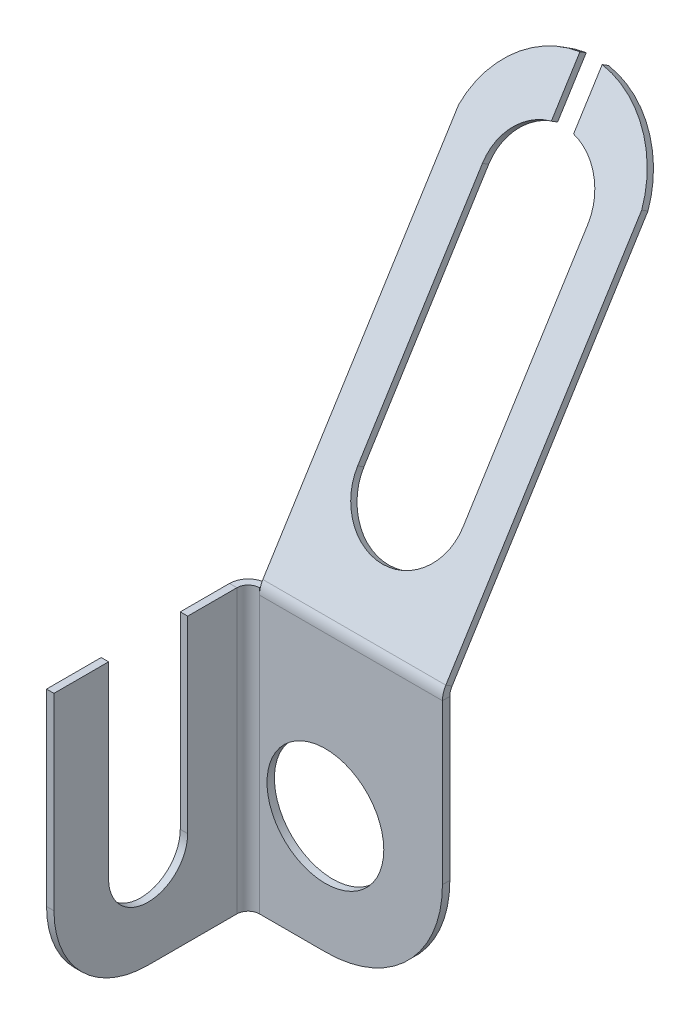
ISO-10303-21;
HEADER;
FILE_DESCRIPTION(('STEP AP214'),'2;1');
FILE_NAME('part.step','',(''),(''),'','','');
FILE_SCHEMA(('AUTOMOTIVE_DESIGN { 1 0 10303 214 1 1 1 1 }'));
ENDSEC;
DATA;
#1=APPLICATION_CONTEXT('core data for automotive mechanical design processes');
#2=APPLICATION_PROTOCOL_DEFINITION('international standard','automotive_design',2000,#1);
#3=PRODUCT_CONTEXT('',#1,'mechanical');
#4=PRODUCT('Part','Part','',(#3));
#5=PRODUCT_RELATED_PRODUCT_CATEGORY('part','',(#4));
#6=PRODUCT_DEFINITION_FORMATION('','',#4);
#7=PRODUCT_DEFINITION_CONTEXT('part definition',#1,'design');
#8=PRODUCT_DEFINITION('design','',#6,#7);
#9=PRODUCT_DEFINITION_SHAPE('','',#8);
#10=(LENGTH_UNIT() NAMED_UNIT(*) SI_UNIT(.MILLI.,.METRE.));
#11=(NAMED_UNIT(*) PLANE_ANGLE_UNIT() SI_UNIT($,.RADIAN.));
#12=(NAMED_UNIT(*) SI_UNIT($,.STERADIAN.) SOLID_ANGLE_UNIT());
#13=UNCERTAINTY_MEASURE_WITH_UNIT(LENGTH_MEASURE(1.E-05),#10,'distance_accuracy_value','');
#14=(GEOMETRIC_REPRESENTATION_CONTEXT(3) GLOBAL_UNCERTAINTY_ASSIGNED_CONTEXT((#13)) GLOBAL_UNIT_ASSIGNED_CONTEXT((#10,
#11,#12)) REPRESENTATION_CONTEXT('',''));
#15=CARTESIAN_POINT('',(0.,0.,0.));
#16=DIRECTION('',(0.,0.,1.));
#17=DIRECTION('',(1.,0.,0.));
#18=AXIS2_PLACEMENT_3D('',#15,#16,#17);
#19=CARTESIAN_POINT('',(1.25999999999999,55.0512584693438,-34.2878670812797));
#20=DIRECTION('',(0.,0.5299192642332,0.848048096156429));
#21=DIRECTION('',(0.,-0.848048096156429,0.5299192642332));
#22=AXIS2_PLACEMENT_3D('',#19,#20,#21);
#23=CYLINDRICAL_SURFACE('',#22,12.5);
#24=DIRECTION('',(0.,0.5299192642332,0.848048096156429));
#25=VECTOR('',#24,1.);
#26=CARTESIAN_POINT('',(2.76000000000004,65.5752585787489,-40.8639922091373));
#27=LINE('',#26,#25);
#28=CARTESIAN_POINT('',(2.76000000000004,70.3445319568478,-33.2315593437294));
#29=VERTEX_POINT('',#28);
#30=CARTESIAN_POINT('',(2.76000000000004,70.8744512210809,-32.383511247573));
#31=VERTEX_POINT('',#30);
#32=EDGE_CURVE('E289',#29,#31,#27,.T.);
#33=ORIENTED_EDGE('',*,*,#32,.T.);
#34=CARTESIAN_POINT('',(1.25999999999999,60.3504511116758,-25.8073861197154));
#35=DIRECTION('',(0.,0.5299192642332,0.848048096156429));
#36=DIRECTION('',(0.,-0.848048096156429,0.5299192642332));
#37=AXIS2_PLACEMENT_3D('',#34,#35,#36);
#38=CIRCLE('',#37,12.5);
#39=CARTESIAN_POINT('',(13.5977,62.0531405103318,-26.8713445407565));
#40=VERTEX_POINT('',#39);
#41=EDGE_CURVE('E302',#40,#31,#38,.T.);
#42=ORIENTED_EDGE('',*,*,#41,.F.);
#43=DIRECTION('',(0.,0.5299192642332,0.848048096156429));
#44=VECTOR('',#43,1.);
#45=CARTESIAN_POINT('',(13.5977,56.7539478679998,-35.3518255023207));
#46=LINE('',#45,#44);
#47=CARTESIAN_POINT('',(13.5977,61.5232212460986,-27.7193926369129));
#48=VERTEX_POINT('',#47);
#49=EDGE_CURVE('E310',#48,#40,#46,.T.);
#50=ORIENTED_EDGE('',*,*,#49,.F.);
#51=CARTESIAN_POINT('',(1.25999999999999,59.8205318474426,-26.6554342158718));
#52=DIRECTION('',(0.,0.5299192642332,0.848048096156429));
#53=DIRECTION('',(0.,-0.848048096156429,0.5299192642332));
#54=AXIS2_PLACEMENT_3D('',#51,#52,#53);
#55=CIRCLE('',#54,12.5);
#56=EDGE_CURVE('E314',#48,#29,#55,.T.);
#57=ORIENTED_EDGE('',*,*,#56,.T.);
#58=EDGE_LOOP('',(#33,#42,#50,#57));
#59=FACE_BOUND('',#58,.T.);
#60=ADVANCED_FACE('F103',(#59),#23,.T.);
#61=CARTESIAN_POINT('',(1.25999999999998,53.5052484421712,-33.321812797555));
#62=DIRECTION('',(0.,0.5299192642332,0.848048096156429));
#63=DIRECTION('',(0.,-0.848048096156429,0.5299192642332));
#64=AXIS2_PLACEMENT_3D('',#61,#62,#63);
#65=CYLINDRICAL_SURFACE('',#64,7.112);
#66=CARTESIAN_POINT('',(1.25999999999998,58.8044410845032,-24.8413318359907));
#67=DIRECTION('',(0.,0.5299192642332,0.848048096156429));
#68=DIRECTION('',(0.,-0.848048096156429,0.5299192642332));
#69=AXIS2_PLACEMENT_3D('',#66,#67,#68);
#70=CIRCLE('',#69,7.112);
#71=CARTESIAN_POINT('',(8.37199999999998,58.8044410845032,-24.8413318359907));
#72=VERTEX_POINT('',#71);
#73=CARTESIAN_POINT('',(2.76000000000004,64.7000860873091,-28.5253397079815));
#74=VERTEX_POINT('',#73);
#75=EDGE_CURVE('E504',#72,#74,#70,.T.);
#76=ORIENTED_EDGE('',*,*,#75,.T.);
#77=DIRECTION('',(0.,0.5299192642332,0.848048096156429));
#78=VECTOR('',#77,1.);
#79=CARTESIAN_POINT('',(2.76000000000004,59.4008934449771,-37.0058206695458));
#80=LINE('',#79,#78);
#81=CARTESIAN_POINT('',(2.76000000000004,64.1701668230759,-29.3733878041379));
#82=VERTEX_POINT('',#81);
#83=EDGE_CURVE('E13',#74,#82,#80,.F.);
#84=ORIENTED_EDGE('',*,*,#83,.T.);
#85=CARTESIAN_POINT('',(1.25999999999998,58.27452182027,-25.6893799321472));
#86=DIRECTION('',(0.,0.5299192642332,0.848048096156429));
#87=DIRECTION('',(0.,-0.848048096156429,0.5299192642332));
#88=AXIS2_PLACEMENT_3D('',#85,#86,#87);
#89=CIRCLE('',#88,7.112);
#90=CARTESIAN_POINT('',(8.37199999999998,58.27452182027,-25.6893799321472));
#91=VERTEX_POINT('',#90);
#92=EDGE_CURVE('E489',#91,#82,#89,.T.);
#93=ORIENTED_EDGE('',*,*,#92,.F.);
#94=DIRECTION('',(0.,0.5299192642332,0.848048096156429));
#95=VECTOR('',#94,1.);
#96=CARTESIAN_POINT('',(8.37199999999998,53.5052484421712,-33.321812797555));
#97=LINE('',#96,#95);
#98=EDGE_CURVE('E308',#91,#72,#97,.T.);
#99=ORIENTED_EDGE('',*,*,#98,.T.);
#100=EDGE_LOOP('',(#76,#84,#93,#99));
#101=FACE_BOUND('',#100,.T.);
#102=ADVANCED_FACE('F533',(#101),#65,.F.);
#103=CARTESIAN_POINT('',(0.,5.14329168215875,8.6898758137614));
#104=DIRECTION('',(0.,0.5299192642332,0.848048096156429));
#105=DIRECTION('',(0.,-0.848048096156429,0.5299192642332));
#106=AXIS2_PLACEMENT_3D('',#103,#104,#105);
#107=PLANE('',#106);
#108=DIRECTION('',(0.,0.848048096156429,-0.5299192642332));
#109=VECTOR('',#108,1.);
#110=CARTESIAN_POINT('',(2.76000000000004,70.8744512210809,-32.383511247573));
#111=LINE('',#110,#109);
#112=EDGE_CURVE('E287',#74,#31,#111,.T.);
#113=ORIENTED_EDGE('',*,*,#112,.F.);
#114=ORIENTED_EDGE('',*,*,#75,.F.);
#115=DIRECTION('',(0.,0.848048096156429,-0.5299192642332));
#116=VECTOR('',#115,1.);
#117=CARTESIAN_POINT('',(8.37199999999998,58.8044410845032,-24.8413318359907));
#118=LINE('',#117,#116);
#119=CARTESIAN_POINT('',(8.37199999999999,31.8789140315366,-8.01639519658663));
#120=VERTEX_POINT('',#119);
#121=EDGE_CURVE('E511',#120,#72,#118,.T.);
#122=ORIENTED_EDGE('',*,*,#121,.F.);
#123=CARTESIAN_POINT('',(1.25999999999999,31.8789140315366,-8.01639519658663));
#124=DIRECTION('',(0.,0.5299192642332,0.848048096156429));
#125=DIRECTION('',(0.,-0.848048096156429,0.5299192642332));
#126=AXIS2_PLACEMENT_3D('',#123,#124,#125);
#127=CIRCLE('',#126,7.112);
#128=CARTESIAN_POINT('',(-5.85200000000001,31.8789140315366,-8.01639519658663));
#129=VERTEX_POINT('',#128);
#130=EDGE_CURVE('E512',#129,#120,#127,.T.);
#131=ORIENTED_EDGE('',*,*,#130,.F.);
#132=DIRECTION('',(0.,-0.848048096156429,0.5299192642332));
#133=VECTOR('',#132,1.);
#134=CARTESIAN_POINT('',(-5.85200000000002,58.8044410845032,-24.8413318359907));
#135=LINE('',#134,#133);
#136=CARTESIAN_POINT('',(-5.85200000000002,58.8044410845032,-24.8413318359907));
#137=VERTEX_POINT('',#136);
#138=EDGE_CURVE('E507',#137,#129,#135,.T.);
#139=ORIENTED_EDGE('',*,*,#138,.F.);
#140=CARTESIAN_POINT('',(-0.239999999999953,64.7000860873091,-28.5253397079815));
#141=VERTEX_POINT('',#140);
#142=EDGE_CURVE('E296',#141,#137,#70,.T.);
#143=ORIENTED_EDGE('',*,*,#142,.F.);
#144=DIRECTION('',(0.,-0.848048096156429,0.5299192642332));
#145=VECTOR('',#144,1.);
#146=CARTESIAN_POINT('',(-0.239999999999957,70.874451221081,-32.383511247573));
#147=LINE('',#146,#145);
#148=CARTESIAN_POINT('',(-0.239999999999957,70.874451221081,-32.383511247573));
#149=VERTEX_POINT('',#148);
#150=EDGE_CURVE('E124',#149,#141,#147,.T.);
#151=ORIENTED_EDGE('',*,*,#150,.F.);
#152=CARTESIAN_POINT('',(-11.0777,62.0531405103319,-26.8713445407565));
#153=VERTEX_POINT('',#152);
#154=EDGE_CURVE('E294',#149,#153,#38,.T.);
#155=ORIENTED_EDGE('',*,*,#154,.T.);
#156=DIRECTION('',(0.,0.848048096156429,-0.5299192642332));
#157=VECTOR('',#156,1.);
#158=CARTESIAN_POINT('',(-11.0777,70.9510523136312,-32.4313769226304));
#159=LINE('',#158,#157);
#160=CARTESIAN_POINT('',(-11.0777,19.7795216354232,-0.455855711530713));
#161=VERTEX_POINT('',#160);
#162=EDGE_CURVE('E325',#161,#153,#159,.T.);
#163=ORIENTED_EDGE('',*,*,#162,.F.);
#164=DIRECTION('',(1.,0.,0.));
#165=VECTOR('',#164,1.);
#166=CARTESIAN_POINT('',(0.,19.7795216354232,-0.455855711530716));
#167=LINE('',#166,#165);
#168=CARTESIAN_POINT('',(13.5977,19.7795216354232,-0.455855711530714));
#169=VERTEX_POINT('',#168);
#170=EDGE_CURVE('E329',#161,#169,#167,.T.);
#171=ORIENTED_EDGE('',*,*,#170,.T.);
#172=DIRECTION('',(0.,-0.848048096156429,0.5299192642332));
#173=VECTOR('',#172,1.);
#174=CARTESIAN_POINT('',(13.5977,19.2931738784744,-0.151951903843572));
#175=LINE('',#174,#173);
#176=EDGE_CURVE('E316',#40,#169,#175,.T.);
#177=ORIENTED_EDGE('',*,*,#176,.F.);
#178=ORIENTED_EDGE('',*,*,#41,.T.);
#179=EDGE_LOOP('',(#113,#114,#122,#131,#139,#143,#151,#155,#163,#171,#177,#178));
#180=FACE_BOUND('',#179,.T.);
#181=ADVANCED_FACE('F291',(#180),#107,.T.);
#182=CARTESIAN_POINT('',(0.,4.61337241792555,7.84182771760497));
#183=DIRECTION('',(0.,0.5299192642332,0.848048096156429));
#184=DIRECTION('',(0.,-0.848048096156429,0.5299192642332));
#185=AXIS2_PLACEMENT_3D('',#182,#183,#184);
#186=PLANE('',#185);
#187=ORIENTED_EDGE('',*,*,#92,.T.);
#188=DIRECTION('',(0.,0.848048096156429,-0.5299192642332));
#189=VECTOR('',#188,1.);
#190=CARTESIAN_POINT('',(2.76000000000004,4.61337241792555,7.84182771760497));
#191=LINE('',#190,#189);
#192=EDGE_CURVE('E116',#82,#29,#191,.T.);
#193=ORIENTED_EDGE('',*,*,#192,.T.);
#194=ORIENTED_EDGE('',*,*,#56,.F.);
#195=DIRECTION('',(0.,0.848048096156429,-0.5299192642332));
#196=VECTOR('',#195,1.);
#197=CARTESIAN_POINT('',(13.5977,4.61337241792555,7.84182771760497));
#198=LINE('',#197,#196);
#199=CARTESIAN_POINT('',(13.5977,19.24960237119,-1.30390380768714));
#200=VERTEX_POINT('',#199);
#201=EDGE_CURVE('E323',#48,#200,#198,.F.);
#202=ORIENTED_EDGE('',*,*,#201,.T.);
#203=DIRECTION('',(-1.,0.,0.));
#204=VECTOR('',#203,1.);
#205=CARTESIAN_POINT('',(-11.0777,19.24960237119,-1.30390380768714));
#206=LINE('',#205,#204);
#207=CARTESIAN_POINT('',(-11.0777,19.24960237119,-1.30390380768714));
#208=VERTEX_POINT('',#207);
#209=EDGE_CURVE('E334',#208,#200,#206,.F.);
#210=ORIENTED_EDGE('',*,*,#209,.F.);
#211=DIRECTION('',(0.,-0.848048096156429,0.5299192642332));
#212=VECTOR('',#211,1.);
#213=CARTESIAN_POINT('',(-11.0777,4.61337241792555,7.84182771760497));
#214=LINE('',#213,#212);
#215=CARTESIAN_POINT('',(-11.0777,61.5232212460987,-27.7193926369129));
#216=VERTEX_POINT('',#215);
#217=EDGE_CURVE('E328',#208,#216,#214,.F.);
#218=ORIENTED_EDGE('',*,*,#217,.T.);
#219=CARTESIAN_POINT('',(-0.239999999999957,70.3445319568478,-33.2315593437294));
#220=VERTEX_POINT('',#219);
#221=EDGE_CURVE('E313',#220,#216,#55,.T.);
#222=ORIENTED_EDGE('',*,*,#221,.F.);
#223=DIRECTION('',(0.,-0.848048096156429,0.5299192642332));
#224=VECTOR('',#223,1.);
#225=CARTESIAN_POINT('',(-0.239999999999957,4.61337241792555,7.84182771760497));
#226=LINE('',#225,#224);
#227=CARTESIAN_POINT('',(-0.239999999999952,64.1701668230759,-29.3733878041379));
#228=VERTEX_POINT('',#227);
#229=EDGE_CURVE('E282',#220,#228,#226,.T.);
#230=ORIENTED_EDGE('',*,*,#229,.T.);
#231=CARTESIAN_POINT('',(-5.85200000000002,58.27452182027,-25.6893799321471));
#232=VERTEX_POINT('',#231);
#233=EDGE_CURVE('E490',#228,#232,#89,.T.);
#234=ORIENTED_EDGE('',*,*,#233,.T.);
#235=DIRECTION('',(0.,-0.848048096156429,0.5299192642332));
#236=VECTOR('',#235,1.);
#237=CARTESIAN_POINT('',(-5.852,4.61337241792555,7.84182771760497));
#238=LINE('',#237,#236);
#239=CARTESIAN_POINT('',(-5.85200000000001,31.3489947673034,-8.86444329274306));
#240=VERTEX_POINT('',#239);
#241=EDGE_CURVE('E476',#232,#240,#238,.T.);
#242=ORIENTED_EDGE('',*,*,#241,.T.);
#243=CARTESIAN_POINT('',(1.25999999999999,31.3489947673034,-8.86444329274305));
#244=DIRECTION('',(0.,0.5299192642332,0.848048096156429));
#245=DIRECTION('',(0.,-0.848048096156429,0.5299192642332));
#246=AXIS2_PLACEMENT_3D('',#243,#244,#245);
#247=CIRCLE('',#246,7.112);
#248=CARTESIAN_POINT('',(8.37199999999999,31.3489947673034,-8.86444329274306));
#249=VERTEX_POINT('',#248);
#250=EDGE_CURVE('E482',#240,#249,#247,.T.);
#251=ORIENTED_EDGE('',*,*,#250,.T.);
#252=DIRECTION('',(0.,0.848048096156429,-0.5299192642332));
#253=VECTOR('',#252,1.);
#254=CARTESIAN_POINT('',(8.372,4.61337241792555,7.84182771760497));
#255=LINE('',#254,#253);
#256=EDGE_CURVE('E488',#249,#91,#255,.T.);
#257=ORIENTED_EDGE('',*,*,#256,.T.);
#258=EDGE_LOOP('',(#187,#193,#194,#202,#210,#218,#222,#230,#234,#242,#251,#257));
#259=FACE_BOUND('',#258,.T.);
#260=ADVANCED_FACE('F498',(#259),#186,.F.);
#261=CARTESIAN_POINT('',(-11.0777,70.9510523136312,-32.4313769226304));
#262=DIRECTION('',(-1.,0.,0.));
#263=DIRECTION('',(0.,-1.,0.));
#264=AXIS2_PLACEMENT_3D('',#261,#262,#263);
#265=PLANE('',#264);
#266=ORIENTED_EDGE('',*,*,#162,.T.);
#267=DIRECTION('',(0.,0.5299192642332,0.848048096156429));
#268=VECTOR('',#267,1.);
#269=CARTESIAN_POINT('',(-11.0777,56.7539478679999,-35.3518255023208));
#270=LINE('',#269,#268);
#271=EDGE_CURVE('E305',#216,#153,#270,.T.);
#272=ORIENTED_EDGE('',*,*,#271,.F.);
#273=ORIENTED_EDGE('',*,*,#217,.F.);
#274=DIRECTION('',(0.,0.5299192642332,0.848048096156429));
#275=VECTOR('',#274,1.);
#276=CARTESIAN_POINT('',(-11.0777,19.7795216354232,-0.455855711530714));
#277=LINE('',#276,#275);
#278=EDGE_CURVE('E319',#208,#161,#277,.T.);
#279=ORIENTED_EDGE('',*,*,#278,.T.);
#280=EDGE_LOOP('',(#266,#272,#273,#279));
#281=FACE_BOUND('',#280,.T.);
#282=ADVANCED_FACE('F892',(#281),#265,.T.);
#283=CARTESIAN_POINT('',(13.5977,19.2931738784744,-0.151951903843572));
#284=DIRECTION('',(1.,0.,0.));
#285=DIRECTION('',(0.,1.,0.));
#286=AXIS2_PLACEMENT_3D('',#283,#284,#285);
#287=PLANE('',#286);
#288=ORIENTED_EDGE('',*,*,#201,.F.);
#289=ORIENTED_EDGE('',*,*,#49,.T.);
#290=ORIENTED_EDGE('',*,*,#176,.T.);
#291=DIRECTION('',(0.,0.5299192642332,0.848048096156429));
#292=VECTOR('',#291,1.);
#293=CARTESIAN_POINT('',(13.5977,19.24960237119,-1.30390380768714));
#294=LINE('',#293,#292);
#295=EDGE_CURVE('E335',#200,#169,#294,.T.);
#296=ORIENTED_EDGE('',*,*,#295,.F.);
#297=EDGE_LOOP('',(#288,#289,#290,#296));
#298=FACE_BOUND('',#297,.T.);
#299=ADVANCED_FACE('F542',(#298),#287,.T.);
#300=CARTESIAN_POINT('',(-11.0777,18.1897638427236,-1.));
#301=DIRECTION('',(1.,0.,0.));
#302=DIRECTION('',(0.,0.,-1.));
#303=AXIS2_PLACEMENT_3D('',#300,#301,#302);
#304=PLANE('',#303);
#305=DIRECTION('',(0.,-1.,0.));
#306=VECTOR('',#305,1.);
#307=CARTESIAN_POINT('',(-11.0777,-19.05,0.));
#308=LINE('',#307,#306);
#309=CARTESIAN_POINT('',(-11.0777,18.1897638427236,0.));
#310=VERTEX_POINT('',#309);
#311=CARTESIAN_POINT('',(-11.0777,19.05,0.));
#312=VERTEX_POINT('',#311);
#313=EDGE_CURVE('E441',#310,#312,#308,.F.);
#314=ORIENTED_EDGE('',*,*,#313,.F.);
#315=CARTESIAN_POINT('',(-11.0777,18.1897638427236,-3.));
#316=DIRECTION('',(1.,0.,0.));
#317=DIRECTION('',(0.,0.,-1.));
#318=AXIS2_PLACEMENT_3D('',#315,#316,#317);
#319=CIRCLE('',#318,3.);
#320=CARTESIAN_POINT('',(-11.0777,19.05,-0.1259795140406));
#321=VERTEX_POINT('',#320);
#322=EDGE_CURVE('E344',#310,#321,#319,.F.);
#323=ORIENTED_EDGE('',*,*,#322,.T.);
#324=DIRECTION('',(0.,0.,-1.));
#325=VECTOR('',#324,1.);
#326=CARTESIAN_POINT('',(-11.0777,19.05,0.));
#327=LINE('',#326,#325);
#328=EDGE_CURVE('E443',#312,#321,#327,.T.);
#329=ORIENTED_EDGE('',*,*,#328,.F.);
#330=EDGE_LOOP('',(#314,#323,#329));
#331=FACE_BOUND('',#330,.T.);
#332=ADVANCED_FACE('F567',(#331),#304,.T.);
#333=CARTESIAN_POINT('',(-2.1503,-3.30200000000001,-1.));
#334=DIRECTION('',(0.,0.,1.));
#335=DIRECTION('',(1.,0.,0.));
#336=AXIS2_PLACEMENT_3D('',#333,#334,#335);
#337=PLANE('',#336);
#338=CARTESIAN_POINT('',(-2.18630000000001,-3.176,-0.999999999999999));
#339=DIRECTION('',(0.,0.,1.));
#340=DIRECTION('',(1.,0.,0.));
#341=AXIS2_PLACEMENT_3D('',#338,#339,#340);
#342=CIRCLE('',#341,7.874);
#343=CARTESIAN_POINT('',(5.68769999999999,-3.176,-0.999999999999999));
#344=VERTEX_POINT('',#343);
#345=EDGE_CURVE('E387',#344,#344,#342,.T.);
#346=ORIENTED_EDGE('',*,*,#345,.T.);
#347=EDGE_LOOP('',(#346));
#348=FACE_BOUND('',#347,.T.);
#349=DIRECTION('',(1.,0.,0.));
#350=VECTOR('',#349,1.);
#351=CARTESIAN_POINT('',(13.5977,18.1897638427236,-1.));
#352=LINE('',#351,#350);
#353=CARTESIAN_POINT('',(13.5977,18.1897638427236,-1.));
#354=VERTEX_POINT('',#353);
#355=CARTESIAN_POINT('',(-11.0777,18.1897638427236,-1.));
#356=VERTEX_POINT('',#355);
#357=EDGE_CURVE('E352',#354,#356,#352,.F.);
#358=ORIENTED_EDGE('',*,*,#357,.F.);
#359=DIRECTION('',(0.,1.,0.));
#360=VECTOR('',#359,1.);
#361=CARTESIAN_POINT('',(13.5977,-3.3019999999999,-1.));
#362=LINE('',#361,#360);
#363=CARTESIAN_POINT('',(13.5977,-3.30200000000001,-1.));
#364=VERTEX_POINT('',#363);
#365=EDGE_CURVE('E451',#364,#354,#362,.T.);
#366=ORIENTED_EDGE('',*,*,#365,.F.);
#367=CARTESIAN_POINT('',(-2.1503,-3.30200000000001,-1.));
#368=DIRECTION('',(0.,0.,1.));
#369=DIRECTION('',(1.,0.,0.));
#370=AXIS2_PLACEMENT_3D('',#367,#368,#369);
#371=CIRCLE('',#370,15.748);
#372=CARTESIAN_POINT('',(-2.15030000000012,-19.05,-1.));
#373=VERTEX_POINT('',#372);
#374=EDGE_CURVE('E460',#373,#364,#371,.T.);
#375=ORIENTED_EDGE('',*,*,#374,.F.);
#376=DIRECTION('',(1.,0.,0.));
#377=VECTOR('',#376,1.);
#378=CARTESIAN_POINT('',(-13.5977,-19.05,-1.));
#379=LINE('',#378,#377);
#380=CARTESIAN_POINT('',(-11.0777,-19.05,-0.999999999999998));
#381=VERTEX_POINT('',#380);
#382=EDGE_CURVE('E453',#381,#373,#379,.T.);
#383=ORIENTED_EDGE('',*,*,#382,.F.);
#384=DIRECTION('',(0.,-1.,0.));
#385=VECTOR('',#384,1.);
#386=CARTESIAN_POINT('',(-11.0777,-19.05,-0.999999999999998));
#387=LINE('',#386,#385);
#388=EDGE_CURVE('E424',#381,#356,#387,.F.);
#389=ORIENTED_EDGE('',*,*,#388,.T.);
#390=EDGE_LOOP('',(#358,#366,#375,#383,#389));
#391=FACE_BOUND('',#390,.T.);
#392=ADVANCED_FACE('F582',(#348,#391),#337,.F.);
#393=CARTESIAN_POINT('',(-2.1503,-3.30200000000001,0.));
#394=DIRECTION('',(0.,0.,1.));
#395=DIRECTION('',(1.,0.,0.));
#396=AXIS2_PLACEMENT_3D('',#393,#394,#395);
#397=PLANE('',#396);
#398=CARTESIAN_POINT('',(-2.18630000000001,-3.176,0.));
#399=DIRECTION('',(0.,0.,1.));
#400=DIRECTION('',(1.,0.,0.));
#401=AXIS2_PLACEMENT_3D('',#398,#399,#400);
#402=CIRCLE('',#401,7.874);
#403=CARTESIAN_POINT('',(5.68769999999999,-3.176,0.));
#404=VERTEX_POINT('',#403);
#405=EDGE_CURVE('E383',#404,#404,#402,.T.);
#406=ORIENTED_EDGE('',*,*,#405,.F.);
#407=EDGE_LOOP('',(#406));
#408=FACE_BOUND('',#407,.T.);
#409=DIRECTION('',(0.,1.,0.));
#410=VECTOR('',#409,1.);
#411=CARTESIAN_POINT('',(13.5977,-3.3019999999999,0.));
#412=LINE('',#411,#410);
#413=CARTESIAN_POINT('',(13.5977,-3.30200000000001,0.));
#414=VERTEX_POINT('',#413);
#415=CARTESIAN_POINT('',(13.5977,18.1897638427236,0.));
#416=VERTEX_POINT('',#415);
#417=EDGE_CURVE('E450',#414,#416,#412,.T.);
#418=ORIENTED_EDGE('',*,*,#417,.T.);
#419=DIRECTION('',(1.,0.,0.));
#420=VECTOR('',#419,1.);
#421=CARTESIAN_POINT('',(13.5977,18.1897638427236,0.));
#422=LINE('',#421,#420);
#423=EDGE_CURVE('E338',#416,#310,#422,.F.);
#424=ORIENTED_EDGE('',*,*,#423,.T.);
#425=CARTESIAN_POINT('',(-11.0777,-19.05,0.));
#426=VERTEX_POINT('',#425);
#427=EDGE_CURVE('E438',#426,#310,#308,.F.);
#428=ORIENTED_EDGE('',*,*,#427,.F.);
#429=DIRECTION('',(1.,0.,0.));
#430=VECTOR('',#429,1.);
#431=CARTESIAN_POINT('',(-13.5977,-19.05,0.));
#432=LINE('',#431,#430);
#433=CARTESIAN_POINT('',(-2.15030000000012,-19.05,0.));
#434=VERTEX_POINT('',#433);
#435=EDGE_CURVE('E463',#426,#434,#432,.T.);
#436=ORIENTED_EDGE('',*,*,#435,.T.);
#437=CARTESIAN_POINT('',(-2.1503,-3.30200000000001,0.));
#438=DIRECTION('',(0.,0.,1.));
#439=DIRECTION('',(1.,0.,0.));
#440=AXIS2_PLACEMENT_3D('',#437,#438,#439);
#441=CIRCLE('',#440,15.748);
#442=EDGE_CURVE('E454',#434,#414,#441,.T.);
#443=ORIENTED_EDGE('',*,*,#442,.T.);
#444=EDGE_LOOP('',(#418,#424,#428,#436,#443));
#445=FACE_BOUND('',#444,.T.);
#446=ADVANCED_FACE('F561',(#408,#445),#397,.T.);
#447=CARTESIAN_POINT('',(13.5977,-3.3019999999999,-1.));
#448=DIRECTION('',(1.,0.,0.));
#449=DIRECTION('',(0.,0.,-1.));
#450=AXIS2_PLACEMENT_3D('',#447,#448,#449);
#451=PLANE('',#450);
#452=ORIENTED_EDGE('',*,*,#365,.T.);
#453=DIRECTION('',(0.,0.,1.));
#454=VECTOR('',#453,1.);
#455=CARTESIAN_POINT('',(13.5977,18.1897638427236,-1.));
#456=LINE('',#455,#454);
#457=EDGE_CURVE('E349',#354,#416,#456,.T.);
#458=ORIENTED_EDGE('',*,*,#457,.T.);
#459=ORIENTED_EDGE('',*,*,#417,.F.);
#460=DIRECTION('',(0.,0.,1.));
#461=VECTOR('',#460,1.);
#462=CARTESIAN_POINT('',(13.5977,-3.30200000000001,-1.));
#463=LINE('',#462,#461);
#464=EDGE_CURVE('E470',#364,#414,#463,.T.);
#465=ORIENTED_EDGE('',*,*,#464,.F.);
#466=EDGE_LOOP('',(#452,#458,#459,#465));
#467=FACE_BOUND('',#466,.T.);
#468=ADVANCED_FACE('F560',(#467),#451,.T.);
#469=CARTESIAN_POINT('',(-13.5977000000001,19.05,26.1954));
#470=DIRECTION('',(0.,1.,0.));
#471=DIRECTION('',(0.,0.,1.));
#472=AXIS2_PLACEMENT_3D('',#469,#470,#471);
#473=PLANE('',#472);
#474=DIRECTION('',(1.,0.,0.));
#475=VECTOR('',#474,1.);
#476=CARTESIAN_POINT('',(-22.5977000000001,19.05,18.8294));
#477=LINE('',#476,#475);
#478=CARTESIAN_POINT('',(-13.5977000000001,19.05,18.8294));
#479=VERTEX_POINT('',#478);
#480=CARTESIAN_POINT('',(-12.5977000000001,19.05,18.8294));
#481=VERTEX_POINT('',#480);
#482=EDGE_CURVE('E373',#479,#481,#477,.T.);
#483=ORIENTED_EDGE('',*,*,#482,.F.);
#484=DIRECTION('',(0.,0.,1.));
#485=VECTOR('',#484,1.);
#486=CARTESIAN_POINT('',(-13.5977000000001,19.05,26.1954));
#487=LINE('',#486,#485);
#488=CARTESIAN_POINT('',(-13.5977000000001,19.05,26.1954));
#489=VERTEX_POINT('',#488);
#490=EDGE_CURVE('E404',#479,#489,#487,.T.);
#491=ORIENTED_EDGE('',*,*,#490,.T.);
#492=DIRECTION('',(1.,0.,0.));
#493=VECTOR('',#492,1.);
#494=CARTESIAN_POINT('',(-13.5977000000001,19.05,26.1954));
#495=LINE('',#494,#493);
#496=CARTESIAN_POINT('',(-12.5977000000001,19.05,26.1954));
#497=VERTEX_POINT('',#496);
#498=EDGE_CURVE('E395',#489,#497,#495,.T.);
#499=ORIENTED_EDGE('',*,*,#498,.T.);
#500=DIRECTION('',(0.,0.,-1.));
#501=VECTOR('',#500,1.);
#502=CARTESIAN_POINT('',(-12.5977,19.05,0.));
#503=LINE('',#502,#501);
#504=EDGE_CURVE('E412',#481,#497,#503,.F.);
#505=ORIENTED_EDGE('',*,*,#504,.F.);
#506=EDGE_LOOP('',(#483,#491,#499,#505));
#507=FACE_BOUND('',#506,.T.);
#508=ADVANCED_FACE('F624',(#507),#473,.T.);
#509=CARTESIAN_POINT('',(-13.5977,-19.05,-1.));
#510=DIRECTION('',(0.,-1.,0.));
#511=DIRECTION('',(0.,0.,-1.));
#512=AXIS2_PLACEMENT_3D('',#509,#510,#511);
#513=PLANE('',#512);
#514=ORIENTED_EDGE('',*,*,#435,.F.);
#515=DIRECTION('',(0.,0.,-1.));
#516=VECTOR('',#515,1.);
#517=CARTESIAN_POINT('',(-11.0777,-19.05,0.));
#518=LINE('',#517,#516);
#519=EDGE_CURVE('E435',#426,#381,#518,.T.);
#520=ORIENTED_EDGE('',*,*,#519,.T.);
#521=ORIENTED_EDGE('',*,*,#382,.T.);
#522=DIRECTION('',(0.,0.,1.));
#523=VECTOR('',#522,1.);
#524=CARTESIAN_POINT('',(-2.15030000000012,-19.05,-1.));
#525=LINE('',#524,#523);
#526=EDGE_CURVE('E457',#373,#434,#525,.T.);
#527=ORIENTED_EDGE('',*,*,#526,.T.);
#528=EDGE_LOOP('',(#514,#520,#521,#527));
#529=FACE_BOUND('',#528,.T.);
#530=ADVANCED_FACE('F589',(#529),#513,.T.);
#531=CARTESIAN_POINT('',(-2.1503,-3.30200000000001,-1.));
#532=DIRECTION('',(0.,0.,1.));
#533=DIRECTION('',(1.,0.,0.));
#534=AXIS2_PLACEMENT_3D('',#531,#532,#533);
#535=CYLINDRICAL_SURFACE('',#534,15.748);
#536=ORIENTED_EDGE('',*,*,#442,.F.);
#537=ORIENTED_EDGE('',*,*,#526,.F.);
#538=ORIENTED_EDGE('',*,*,#374,.T.);
#539=ORIENTED_EDGE('',*,*,#464,.T.);
#540=EDGE_LOOP('',(#536,#537,#538,#539));
#541=FACE_BOUND('',#540,.T.);
#542=ADVANCED_FACE('F692',(#541),#535,.T.);
#543=CARTESIAN_POINT('',(-11.0777,19.05,1.52));
#544=DIRECTION('',(0.,1.,0.));
#545=DIRECTION('',(0.,0.,1.));
#546=AXIS2_PLACEMENT_3D('',#543,#544,#545);
#547=PLANE('',#546);
#548=DIRECTION('',(-1.,0.,0.));
#549=VECTOR('',#548,1.);
#550=CARTESIAN_POINT('',(-13.5977,19.05,1.51999999999999));
#551=LINE('',#550,#549);
#552=CARTESIAN_POINT('',(-12.5977,19.05,1.51999999999999));
#553=VERTEX_POINT('',#552);
#554=CARTESIAN_POINT('',(-13.5977,19.05,1.51999999999999));
#555=VERTEX_POINT('',#554);
#556=EDGE_CURVE('E393',#553,#555,#551,.T.);
#557=ORIENTED_EDGE('',*,*,#556,.F.);
#558=CARTESIAN_POINT('',(-11.0777,19.05,1.52));
#559=DIRECTION('',(0.,-1.,0.));
#560=DIRECTION('',(0.,0.,-1.));
#561=AXIS2_PLACEMENT_3D('',#558,#559,#560);
#562=CIRCLE('',#561,1.52);
#563=EDGE_CURVE('E434',#312,#553,#562,.F.);
#564=ORIENTED_EDGE('',*,*,#563,.F.);
#565=ORIENTED_EDGE('',*,*,#328,.T.);
#566=CARTESIAN_POINT('',(-11.0777,19.05,-1.));
#567=VERTEX_POINT('',#566);
#568=EDGE_CURVE('E449',#321,#567,#327,.T.);
#569=ORIENTED_EDGE('',*,*,#568,.T.);
#570=CARTESIAN_POINT('',(-11.0777,19.05,1.52));
#571=DIRECTION('',(0.,-1.,0.));
#572=DIRECTION('',(0.,0.,-1.));
#573=AXIS2_PLACEMENT_3D('',#570,#571,#572);
#574=CIRCLE('',#573,2.52);
#575=EDGE_CURVE('E426',#567,#555,#574,.F.);
#576=ORIENTED_EDGE('',*,*,#575,.T.);
#577=EDGE_LOOP('',(#557,#564,#565,#569,#576));
#578=FACE_BOUND('',#577,.T.);
#579=ADVANCED_FACE('F574',(#578),#547,.T.);
#580=CARTESIAN_POINT('',(-11.0777,-19.05,1.52));
#581=DIRECTION('',(0.,1.,0.));
#582=DIRECTION('',(0.,0.,1.));
#583=AXIS2_PLACEMENT_3D('',#580,#581,#582);
#584=PLANE('',#583);
#585=CARTESIAN_POINT('',(-11.0777,-19.05,1.52));
#586=DIRECTION('',(0.,-1.,0.));
#587=DIRECTION('',(0.,0.,-1.));
#588=AXIS2_PLACEMENT_3D('',#585,#586,#587);
#589=CIRCLE('',#588,1.52);
#590=CARTESIAN_POINT('',(-12.5977,-19.05,1.52));
#591=VERTEX_POINT('',#590);
#592=EDGE_CURVE('E392',#591,#426,#589,.T.);
#593=ORIENTED_EDGE('',*,*,#592,.F.);
#594=DIRECTION('',(-1.,0.,0.));
#595=VECTOR('',#594,1.);
#596=CARTESIAN_POINT('',(-12.5977,-19.05,1.52));
#597=LINE('',#596,#595);
#598=CARTESIAN_POINT('',(-13.5977,-19.05,1.51999999999999));
#599=VERTEX_POINT('',#598);
#600=EDGE_CURVE('E419',#591,#599,#597,.T.);
#601=ORIENTED_EDGE('',*,*,#600,.T.);
#602=CARTESIAN_POINT('',(-11.0777,-19.05,1.52));
#603=DIRECTION('',(0.,-1.,0.));
#604=DIRECTION('',(0.,0.,-1.));
#605=AXIS2_PLACEMENT_3D('',#602,#603,#604);
#606=CIRCLE('',#605,2.52);
#607=EDGE_CURVE('E429',#599,#381,#606,.T.);
#608=ORIENTED_EDGE('',*,*,#607,.T.);
#609=ORIENTED_EDGE('',*,*,#519,.F.);
#610=EDGE_LOOP('',(#593,#601,#608,#609));
#611=FACE_BOUND('',#610,.T.);
#612=ADVANCED_FACE('F595',(#611),#584,.F.);
#613=CARTESIAN_POINT('',(-11.0777,-19.05,1.52));
#614=DIRECTION('',(0.,-1.,0.));
#615=DIRECTION('',(-1.,0.,0.));
#616=AXIS2_PLACEMENT_3D('',#613,#614,#615);
#617=CYLINDRICAL_SURFACE('',#616,2.52);
#618=ORIENTED_EDGE('',*,*,#388,.F.);
#619=ORIENTED_EDGE('',*,*,#607,.F.);
#620=DIRECTION('',(0.,-1.,0.));
#621=VECTOR('',#620,1.);
#622=CARTESIAN_POINT('',(-13.5977,0.,1.51999999999999));
#623=LINE('',#622,#621);
#624=EDGE_CURVE('E415',#555,#599,#623,.T.);
#625=ORIENTED_EDGE('',*,*,#624,.F.);
#626=ORIENTED_EDGE('',*,*,#575,.F.);
#627=DIRECTION('',(0.,1.,0.));
#628=VECTOR('',#627,1.);
#629=CARTESIAN_POINT('',(-11.0777,18.1897638427236,-1.));
#630=LINE('',#629,#628);
#631=EDGE_CURVE('E360',#356,#567,#630,.T.);
#632=ORIENTED_EDGE('',*,*,#631,.F.);
#633=EDGE_LOOP('',(#618,#619,#625,#626,#632));
#634=FACE_BOUND('',#633,.T.);
#635=ADVANCED_FACE('F578',(#634),#617,.T.);
#636=CARTESIAN_POINT('',(-11.0777,-19.05,1.52));
#637=DIRECTION('',(0.,-1.,0.));
#638=DIRECTION('',(-1.,0.,0.));
#639=AXIS2_PLACEMENT_3D('',#636,#637,#638);
#640=CYLINDRICAL_SURFACE('',#639,1.52);
#641=ORIENTED_EDGE('',*,*,#427,.T.);
#642=ORIENTED_EDGE('',*,*,#313,.T.);
#643=ORIENTED_EDGE('',*,*,#563,.T.);
#644=DIRECTION('',(0.,1.,0.));
#645=VECTOR('',#644,1.);
#646=CARTESIAN_POINT('',(-12.5977,19.05,1.52));
#647=LINE('',#646,#645);
#648=EDGE_CURVE('E416',#553,#591,#647,.F.);
#649=ORIENTED_EDGE('',*,*,#648,.T.);
#650=ORIENTED_EDGE('',*,*,#592,.T.);
#651=EDGE_LOOP('',(#641,#642,#643,#649,#650));
#652=FACE_BOUND('',#651,.T.);
#653=ADVANCED_FACE('F594',(#652),#640,.F.);
#654=CARTESIAN_POINT('',(-13.5977,-19.05,0.));
#655=DIRECTION('',(0.,-1.,0.));
#656=DIRECTION('',(0.,0.,-1.));
#657=AXIS2_PLACEMENT_3D('',#654,#655,#656);
#658=PLANE('',#657);
#659=DIRECTION('',(0.,0.,1.));
#660=VECTOR('',#659,1.);
#661=CARTESIAN_POINT('',(-12.5977,-19.05,0.));
#662=LINE('',#661,#660);
#663=CARTESIAN_POINT('',(-12.5977000000001,-19.05,13.4954));
#664=VERTEX_POINT('',#663);
#665=EDGE_CURVE('E403',#664,#591,#662,.F.);
#666=ORIENTED_EDGE('',*,*,#665,.F.);
#667=DIRECTION('',(1.,0.,0.));
#668=VECTOR('',#667,1.);
#669=CARTESIAN_POINT('',(-13.5977000000001,-19.05,13.4954));
#670=LINE('',#669,#668);
#671=CARTESIAN_POINT('',(-13.5977000000001,-19.05,13.4954));
#672=VERTEX_POINT('',#671);
#673=EDGE_CURVE('E478',#664,#672,#670,.F.);
#674=ORIENTED_EDGE('',*,*,#673,.T.);
#675=DIRECTION('',(0.,0.,-1.));
#676=VECTOR('',#675,1.);
#677=CARTESIAN_POINT('',(-13.5977,-19.05,0.));
#678=LINE('',#677,#676);
#679=EDGE_CURVE('E396',#672,#599,#678,.T.);
#680=ORIENTED_EDGE('',*,*,#679,.T.);
#681=ORIENTED_EDGE('',*,*,#600,.F.);
#682=EDGE_LOOP('',(#666,#674,#680,#681));
#683=FACE_BOUND('',#682,.T.);
#684=ADVANCED_FACE('F632',(#683),#658,.T.);
#685=DIRECTION('',(1.,0.,0.));
#686=VECTOR('',#685,1.);
#687=CARTESIAN_POINT('',(-22.5977,19.05,8.16139999999997));
#688=LINE('',#687,#686);
#689=CARTESIAN_POINT('',(-13.5977,19.05,8.1614));
#690=VERTEX_POINT('',#689);
#691=CARTESIAN_POINT('',(-12.5977,19.05,8.16140000000001));
#692=VERTEX_POINT('',#691);
#693=EDGE_CURVE('E374',#690,#692,#688,.T.);
#694=ORIENTED_EDGE('',*,*,#693,.T.);
#695=EDGE_CURVE('E409',#553,#692,#503,.F.);
#696=ORIENTED_EDGE('',*,*,#695,.F.);
#697=ORIENTED_EDGE('',*,*,#556,.T.);
#698=EDGE_CURVE('E402',#555,#690,#487,.T.);
#699=ORIENTED_EDGE('',*,*,#698,.T.);
#700=EDGE_LOOP('',(#694,#696,#697,#699));
#701=FACE_BOUND('',#700,.T.);
#702=ADVANCED_FACE('F603',(#701),#473,.T.);
#703=CARTESIAN_POINT('',(-13.5977,0.,0.));
#704=DIRECTION('',(-1.,0.,0.));
#705=DIRECTION('',(0.,0.,1.));
#706=AXIS2_PLACEMENT_3D('',#703,#704,#705);
#707=PLANE('',#706);
#708=DIRECTION('',(0.,1.,0.));
#709=VECTOR('',#708,1.);
#710=CARTESIAN_POINT('',(-13.5977000000001,0.,18.8294));
#711=LINE('',#710,#709);
#712=CARTESIAN_POINT('',(-13.5977000000001,-6.35,18.8294));
#713=VERTEX_POINT('',#712);
#714=EDGE_CURVE('E382',#713,#479,#711,.T.);
#715=ORIENTED_EDGE('',*,*,#714,.F.);
#716=CARTESIAN_POINT('',(-13.5977000000001,-6.35,13.4954));
#717=DIRECTION('',(-1.,0.,0.));
#718=DIRECTION('',(0.,0.,1.));
#719=AXIS2_PLACEMENT_3D('',#716,#717,#718);
#720=CIRCLE('',#719,5.334);
#721=CARTESIAN_POINT('',(-13.5977,-6.34999999999998,8.1614));
#722=VERTEX_POINT('',#721);
#723=EDGE_CURVE('E384',#722,#713,#720,.T.);
#724=ORIENTED_EDGE('',*,*,#723,.F.);
#725=DIRECTION('',(0.,-1.,0.));
#726=VECTOR('',#725,1.);
#727=CARTESIAN_POINT('',(-13.5977,0.,8.1614));
#728=LINE('',#727,#726);
#729=EDGE_CURVE('E375',#690,#722,#728,.T.);
#730=ORIENTED_EDGE('',*,*,#729,.F.);
#731=ORIENTED_EDGE('',*,*,#698,.F.);
#732=ORIENTED_EDGE('',*,*,#624,.T.);
#733=ORIENTED_EDGE('',*,*,#679,.F.);
#734=CARTESIAN_POINT('',(-13.5977000000001,-6.34999999999999,13.4954));
#735=DIRECTION('',(-1.,0.,0.));
#736=DIRECTION('',(0.,0.,1.));
#737=AXIS2_PLACEMENT_3D('',#734,#735,#736);
#738=CIRCLE('',#737,12.7);
#739=CARTESIAN_POINT('',(-13.5977000000001,-6.34999999999999,26.1954));
#740=VERTEX_POINT('',#739);
#741=EDGE_CURVE('E477',#672,#740,#738,.T.);
#742=ORIENTED_EDGE('',*,*,#741,.T.);
#743=DIRECTION('',(0.,-1.,0.));
#744=VECTOR('',#743,1.);
#745=CARTESIAN_POINT('',(-13.5977000000001,-19.05,26.1954));
#746=LINE('',#745,#744);
#747=EDGE_CURVE('E398',#489,#740,#746,.T.);
#748=ORIENTED_EDGE('',*,*,#747,.F.);
#749=ORIENTED_EDGE('',*,*,#490,.F.);
#750=EDGE_LOOP('',(#715,#724,#730,#731,#732,#733,#742,#748,#749));
#751=FACE_BOUND('',#750,.T.);
#752=ADVANCED_FACE('F612',(#751),#707,.T.);
#753=CARTESIAN_POINT('',(-12.5977,0.,0.));
#754=DIRECTION('',(-1.,0.,0.));
#755=DIRECTION('',(0.,0.,1.));
#756=AXIS2_PLACEMENT_3D('',#753,#754,#755);
#757=PLANE('',#756);
#758=CARTESIAN_POINT('',(-12.5977000000001,-6.35,13.4954));
#759=DIRECTION('',(1.,0.,0.));
#760=DIRECTION('',(0.,0.,-1.));
#761=AXIS2_PLACEMENT_3D('',#758,#759,#760);
#762=CIRCLE('',#761,5.334);
#763=CARTESIAN_POINT('',(-12.5977000000001,-6.35,18.8294));
#764=VERTEX_POINT('',#763);
#765=CARTESIAN_POINT('',(-12.5977,-6.34999999999998,8.1614));
#766=VERTEX_POINT('',#765);
#767=EDGE_CURVE('E365',#764,#766,#762,.T.);
#768=ORIENTED_EDGE('',*,*,#767,.F.);
#769=DIRECTION('',(0.,-1.,0.));
#770=VECTOR('',#769,1.);
#771=CARTESIAN_POINT('',(-12.5977000000001,-6.35,18.8294));
#772=LINE('',#771,#770);
#773=EDGE_CURVE('E366',#481,#764,#772,.T.);
#774=ORIENTED_EDGE('',*,*,#773,.F.);
#775=ORIENTED_EDGE('',*,*,#504,.T.);
#776=DIRECTION('',(0.,1.,0.));
#777=VECTOR('',#776,1.);
#778=CARTESIAN_POINT('',(-12.5977000000001,0.,26.1954));
#779=LINE('',#778,#777);
#780=CARTESIAN_POINT('',(-12.5977000000001,-6.34999999999999,26.1954));
#781=VERTEX_POINT('',#780);
#782=EDGE_CURVE('E410',#497,#781,#779,.F.);
#783=ORIENTED_EDGE('',*,*,#782,.T.);
#784=CARTESIAN_POINT('',(-12.5977000000001,-6.34999999999999,13.4954));
#785=DIRECTION('',(-1.,0.,0.));
#786=DIRECTION('',(0.,0.,1.));
#787=AXIS2_PLACEMENT_3D('',#784,#785,#786);
#788=CIRCLE('',#787,12.7);
#789=EDGE_CURVE('E473',#781,#664,#788,.F.);
#790=ORIENTED_EDGE('',*,*,#789,.T.);
#791=ORIENTED_EDGE('',*,*,#665,.T.);
#792=ORIENTED_EDGE('',*,*,#648,.F.);
#793=ORIENTED_EDGE('',*,*,#695,.T.);
#794=DIRECTION('',(0.,1.,0.));
#795=VECTOR('',#794,1.);
#796=CARTESIAN_POINT('',(-12.5977,-6.34999999999998,8.1614));
#797=LINE('',#796,#795);
#798=EDGE_CURVE('E364',#766,#692,#797,.T.);
#799=ORIENTED_EDGE('',*,*,#798,.F.);
#800=EDGE_LOOP('',(#768,#774,#775,#783,#790,#791,#792,#793,#799));
#801=FACE_BOUND('',#800,.T.);
#802=ADVANCED_FACE('F598',(#801),#757,.F.);
#803=CARTESIAN_POINT('',(-13.5977000000001,-19.05,26.1954));
#804=DIRECTION('',(0.,0.,1.));
#805=DIRECTION('',(1.,0.,0.));
#806=AXIS2_PLACEMENT_3D('',#803,#804,#805);
#807=PLANE('',#806);
#808=ORIENTED_EDGE('',*,*,#747,.T.);
#809=DIRECTION('',(1.,0.,0.));
#810=VECTOR('',#809,1.);
#811=CARTESIAN_POINT('',(-13.5977000000001,-6.34999999999999,26.1954));
#812=LINE('',#811,#810);
#813=EDGE_CURVE('E469',#740,#781,#812,.T.);
#814=ORIENTED_EDGE('',*,*,#813,.T.);
#815=ORIENTED_EDGE('',*,*,#782,.F.);
#816=ORIENTED_EDGE('',*,*,#498,.F.);
#817=EDGE_LOOP('',(#808,#814,#815,#816));
#818=FACE_BOUND('',#817,.T.);
#819=ADVANCED_FACE('F627',(#818),#807,.T.);
#820=CARTESIAN_POINT('',(-13.5977000000001,-6.34999999999999,13.4954));
#821=DIRECTION('',(1.,0.,0.));
#822=DIRECTION('',(0.,0.,-1.));
#823=AXIS2_PLACEMENT_3D('',#820,#821,#822);
#824=CYLINDRICAL_SURFACE('',#823,12.7);
#825=ORIENTED_EDGE('',*,*,#741,.F.);
#826=ORIENTED_EDGE('',*,*,#673,.F.);
#827=ORIENTED_EDGE('',*,*,#789,.F.);
#828=ORIENTED_EDGE('',*,*,#813,.F.);
#829=EDGE_LOOP('',(#825,#826,#827,#828));
#830=FACE_BOUND('',#829,.T.);
#831=ADVANCED_FACE('F101',(#830),#824,.T.);
#832=CARTESIAN_POINT('',(-2.18630000000001,-3.176,-10.));
#833=DIRECTION('',(0.,0.,1.));
#834=DIRECTION('',(1.,0.,0.));
#835=AXIS2_PLACEMENT_3D('',#832,#833,#834);
#836=CYLINDRICAL_SURFACE('',#835,7.874);
#837=ORIENTED_EDGE('',*,*,#405,.T.);
#838=EDGE_LOOP('',(#837));
#839=FACE_BOUND('',#838,.T.);
#840=ORIENTED_EDGE('',*,*,#345,.F.);
#841=EDGE_LOOP('',(#840));
#842=FACE_BOUND('',#841,.T.);
#843=ADVANCED_FACE('F637',(#839,#842),#836,.F.);
#844=CARTESIAN_POINT('',(-22.5977000000001,-6.35,13.4954));
#845=DIRECTION('',(1.,0.,0.));
#846=DIRECTION('',(0.,0.,-1.));
#847=AXIS2_PLACEMENT_3D('',#844,#845,#846);
#848=CYLINDRICAL_SURFACE('',#847,5.334);
#849=ORIENTED_EDGE('',*,*,#723,.T.);
#850=DIRECTION('',(1.,0.,0.));
#851=VECTOR('',#850,1.);
#852=CARTESIAN_POINT('',(-22.5977000000001,-6.35,18.8294));
#853=LINE('',#852,#851);
#854=EDGE_CURVE('E369',#713,#764,#853,.T.);
#855=ORIENTED_EDGE('',*,*,#854,.T.);
#856=ORIENTED_EDGE('',*,*,#767,.T.);
#857=DIRECTION('',(1.,0.,0.));
#858=VECTOR('',#857,1.);
#859=CARTESIAN_POINT('',(-22.5977,-6.34999999999998,8.16139999999997));
#860=LINE('',#859,#858);
#861=EDGE_CURVE('E367',#722,#766,#860,.T.);
#862=ORIENTED_EDGE('',*,*,#861,.F.);
#863=EDGE_LOOP('',(#849,#855,#856,#862));
#864=FACE_BOUND('',#863,.T.);
#865=ADVANCED_FACE('F617',(#864),#848,.F.);
#866=CARTESIAN_POINT('',(-22.5977000000001,-6.35,18.8294));
#867=DIRECTION('',(0.,0.,1.));
#868=DIRECTION('',(1.,0.,0.));
#869=AXIS2_PLACEMENT_3D('',#866,#867,#868);
#870=PLANE('',#869);
#871=ORIENTED_EDGE('',*,*,#714,.T.);
#872=ORIENTED_EDGE('',*,*,#482,.T.);
#873=ORIENTED_EDGE('',*,*,#773,.T.);
#874=ORIENTED_EDGE('',*,*,#854,.F.);
#875=EDGE_LOOP('',(#871,#872,#873,#874));
#876=FACE_BOUND('',#875,.T.);
#877=ADVANCED_FACE('F620',(#876),#870,.F.);
#878=CARTESIAN_POINT('',(-22.5977,-6.34999999999998,8.16139999999997));
#879=DIRECTION('',(0.,0.,-1.));
#880=DIRECTION('',(-1.,0.,0.));
#881=AXIS2_PLACEMENT_3D('',#878,#879,#880);
#882=PLANE('',#881);
#883=ORIENTED_EDGE('',*,*,#729,.T.);
#884=ORIENTED_EDGE('',*,*,#861,.T.);
#885=ORIENTED_EDGE('',*,*,#798,.T.);
#886=ORIENTED_EDGE('',*,*,#693,.F.);
#887=EDGE_LOOP('',(#883,#884,#885,#886));
#888=FACE_BOUND('',#887,.T.);
#889=ADVANCED_FACE('F607',(#888),#882,.F.);
#890=CARTESIAN_POINT('',(-11.0777,18.1897638427236,-3.));
#891=DIRECTION('',(-1.,0.,0.));
#892=DIRECTION('',(0.,0.,1.));
#893=AXIS2_PLACEMENT_3D('',#890,#891,#892);
#894=PLANE('',#893);
#895=ORIENTED_EDGE('',*,*,#568,.F.);
#896=EDGE_CURVE('E342',#321,#161,#319,.F.);
#897=ORIENTED_EDGE('',*,*,#896,.T.);
#898=ORIENTED_EDGE('',*,*,#278,.F.);
#899=CARTESIAN_POINT('',(-11.0777,18.1897638427236,-3.));
#900=DIRECTION('',(1.,0.,0.));
#901=DIRECTION('',(0.,0.,-1.));
#902=AXIS2_PLACEMENT_3D('',#899,#900,#901);
#903=CIRCLE('',#902,2.);
#904=EDGE_CURVE('E346',#356,#208,#903,.F.);
#905=ORIENTED_EDGE('',*,*,#904,.F.);
#906=ORIENTED_EDGE('',*,*,#631,.T.);
#907=EDGE_LOOP('',(#895,#897,#898,#905,#906));
#908=FACE_BOUND('',#907,.T.);
#909=ADVANCED_FACE('F580',(#908),#894,.T.);
#910=CARTESIAN_POINT('',(13.5977,18.1897638427236,-3.));
#911=DIRECTION('',(-1.,0.,0.));
#912=DIRECTION('',(0.,0.,1.));
#913=AXIS2_PLACEMENT_3D('',#910,#911,#912);
#914=PLANE('',#913);
#915=CARTESIAN_POINT('',(13.5977,18.1897638427236,-3.));
#916=DIRECTION('',(1.,0.,0.));
#917=DIRECTION('',(0.,0.,-1.));
#918=AXIS2_PLACEMENT_3D('',#915,#916,#917);
#919=CIRCLE('',#918,2.);
#920=EDGE_CURVE('E321',#200,#354,#919,.T.);
#921=ORIENTED_EDGE('',*,*,#920,.F.);
#922=ORIENTED_EDGE('',*,*,#295,.T.);
#923=CARTESIAN_POINT('',(13.5977,18.1897638427236,-3.));
#924=DIRECTION('',(1.,0.,0.));
#925=DIRECTION('',(0.,0.,-1.));
#926=AXIS2_PLACEMENT_3D('',#923,#924,#925);
#927=CIRCLE('',#926,3.);
#928=EDGE_CURVE('E343',#169,#416,#927,.T.);
#929=ORIENTED_EDGE('',*,*,#928,.T.);
#930=ORIENTED_EDGE('',*,*,#457,.F.);
#931=EDGE_LOOP('',(#921,#922,#929,#930));
#932=FACE_BOUND('',#931,.T.);
#933=ADVANCED_FACE('F555',(#932),#914,.F.);
#934=CARTESIAN_POINT('',(13.5977,18.1897638427236,-3.));
#935=DIRECTION('',(1.,0.,0.));
#936=DIRECTION('',(0.,0.5299192642332,0.848048096156429));
#937=AXIS2_PLACEMENT_3D('',#934,#935,#936);
#938=CYLINDRICAL_SURFACE('',#937,3.);
#939=ORIENTED_EDGE('',*,*,#423,.F.);
#940=ORIENTED_EDGE('',*,*,#928,.F.);
#941=ORIENTED_EDGE('',*,*,#170,.F.);
#942=ORIENTED_EDGE('',*,*,#896,.F.);
#943=ORIENTED_EDGE('',*,*,#322,.F.);
#944=EDGE_LOOP('',(#939,#940,#941,#942,#943));
#945=FACE_BOUND('',#944,.T.);
#946=ADVANCED_FACE('F564',(#945),#938,.T.);
#947=CARTESIAN_POINT('',(13.5977,18.1897638427236,-3.));
#948=DIRECTION('',(1.,0.,0.));
#949=DIRECTION('',(0.,0.5299192642332,0.848048096156429));
#950=AXIS2_PLACEMENT_3D('',#947,#948,#949);
#951=CYLINDRICAL_SURFACE('',#950,2.);
#952=ORIENTED_EDGE('',*,*,#357,.T.);
#953=ORIENTED_EDGE('',*,*,#904,.T.);
#954=ORIENTED_EDGE('',*,*,#209,.T.);
#955=ORIENTED_EDGE('',*,*,#920,.T.);
#956=EDGE_LOOP('',(#952,#953,#954,#955));
#957=FACE_BOUND('',#956,.T.);
#958=ADVANCED_FACE('F546',(#957),#951,.F.);
#959=DIRECTION('',(0.,0.5299192642332,0.848048096156429));
#960=VECTOR('',#959,1.);
#961=CARTESIAN_POINT('',(-0.239999999999957,65.575258578749,-40.8639922091373));
#962=LINE('',#961,#960);
#963=EDGE_CURVE('E279',#220,#149,#962,.T.);
#964=ORIENTED_EDGE('',*,*,#963,.F.);
#965=ORIENTED_EDGE('',*,*,#221,.T.);
#966=ORIENTED_EDGE('',*,*,#271,.T.);
#967=ORIENTED_EDGE('',*,*,#154,.F.);
#968=EDGE_LOOP('',(#964,#965,#966,#967));
#969=FACE_BOUND('',#968,.T.);
#970=ADVANCED_FACE('F297',(#969),#23,.T.);
#971=ORIENTED_EDGE('',*,*,#233,.F.);
#972=DIRECTION('',(0.,0.5299192642332,0.848048096156429));
#973=VECTOR('',#972,1.);
#974=CARTESIAN_POINT('',(-0.239999999999957,59.4008934449771,-37.0058206695458));
#975=LINE('',#974,#973);
#976=EDGE_CURVE('E107',#228,#141,#975,.T.);
#977=ORIENTED_EDGE('',*,*,#976,.T.);
#978=ORIENTED_EDGE('',*,*,#142,.T.);
#979=DIRECTION('',(0.,0.5299192642332,0.848048096156429));
#980=VECTOR('',#979,1.);
#981=CARTESIAN_POINT('',(-5.85200000000002,53.5052484421712,-33.321812797555));
#982=LINE('',#981,#980);
#983=EDGE_CURVE('E520',#232,#137,#982,.T.);
#984=ORIENTED_EDGE('',*,*,#983,.F.);
#985=EDGE_LOOP('',(#971,#977,#978,#984));
#986=FACE_BOUND('',#985,.T.);
#987=ADVANCED_FACE('F494',(#986),#65,.F.);
#988=CARTESIAN_POINT('',(8.37199999999998,53.5052484421712,-33.321812797555));
#989=DIRECTION('',(1.,0.,0.));
#990=DIRECTION('',(0.,1.,0.));
#991=AXIS2_PLACEMENT_3D('',#988,#989,#990);
#992=PLANE('',#991);
#993=DIRECTION('',(0.,0.5299192642332,0.848048096156429));
#994=VECTOR('',#993,1.);
#995=CARTESIAN_POINT('',(8.37199999999999,26.5797213892046,-16.4968761581509));
#996=LINE('',#995,#994);
#997=EDGE_CURVE('E518',#249,#120,#996,.T.);
#998=ORIENTED_EDGE('',*,*,#997,.T.);
#999=ORIENTED_EDGE('',*,*,#121,.T.);
#1000=ORIENTED_EDGE('',*,*,#98,.F.);
#1001=ORIENTED_EDGE('',*,*,#256,.F.);
#1002=EDGE_LOOP('',(#998,#999,#1000,#1001));
#1003=FACE_BOUND('',#1002,.T.);
#1004=ADVANCED_FACE('F531',(#1003),#992,.F.);
#1005=CARTESIAN_POINT('',(1.25999999999999,26.5797213892046,-16.4968761581509));
#1006=DIRECTION('',(0.,0.5299192642332,0.848048096156429));
#1007=DIRECTION('',(0.,-0.848048096156429,0.5299192642332));
#1008=AXIS2_PLACEMENT_3D('',#1005,#1006,#1007);
#1009=CYLINDRICAL_SURFACE('',#1008,7.112);
#1010=DIRECTION('',(0.,0.5299192642332,0.848048096156429));
#1011=VECTOR('',#1010,1.);
#1012=CARTESIAN_POINT('',(-5.85200000000001,26.5797213892046,-16.4968761581509));
#1013=LINE('',#1012,#1011);
#1014=EDGE_CURVE('E523',#240,#129,#1013,.T.);
#1015=ORIENTED_EDGE('',*,*,#1014,.T.);
#1016=ORIENTED_EDGE('',*,*,#130,.T.);
#1017=ORIENTED_EDGE('',*,*,#997,.F.);
#1018=ORIENTED_EDGE('',*,*,#250,.F.);
#1019=EDGE_LOOP('',(#1015,#1016,#1017,#1018));
#1020=FACE_BOUND('',#1019,.T.);
#1021=ADVANCED_FACE('F527',(#1020),#1009,.F.);
#1022=CARTESIAN_POINT('',(-5.85200000000002,53.5052484421712,-33.321812797555));
#1023=DIRECTION('',(-1.,0.,0.));
#1024=DIRECTION('',(0.,-1.,0.));
#1025=AXIS2_PLACEMENT_3D('',#1022,#1023,#1024);
#1026=PLANE('',#1025);
#1027=ORIENTED_EDGE('',*,*,#983,.T.);
#1028=ORIENTED_EDGE('',*,*,#138,.T.);
#1029=ORIENTED_EDGE('',*,*,#1014,.F.);
#1030=ORIENTED_EDGE('',*,*,#241,.F.);
#1031=EDGE_LOOP('',(#1027,#1028,#1029,#1030));
#1032=FACE_BOUND('',#1031,.T.);
#1033=ADVANCED_FACE('F521',(#1032),#1026,.F.);
#1034=CARTESIAN_POINT('',(-0.239999999999957,65.575258578749,-40.8639922091373));
#1035=DIRECTION('',(-1.,0.,0.));
#1036=DIRECTION('',(0.,0.,1.));
#1037=AXIS2_PLACEMENT_3D('',#1034,#1035,#1036);
#1038=PLANE('',#1037);
#1039=ORIENTED_EDGE('',*,*,#963,.T.);
#1040=ORIENTED_EDGE('',*,*,#150,.T.);
#1041=ORIENTED_EDGE('',*,*,#976,.F.);
#1042=ORIENTED_EDGE('',*,*,#229,.F.);
#1043=EDGE_LOOP('',(#1039,#1040,#1041,#1042));
#1044=FACE_BOUND('',#1043,.T.);
#1045=ADVANCED_FACE('F283',(#1044),#1038,.F.);
#1046=CARTESIAN_POINT('',(2.76000000000004,65.5752585787489,-40.8639922091373));
#1047=DIRECTION('',(1.,0.,0.));
#1048=DIRECTION('',(0.,0.,-1.));
#1049=AXIS2_PLACEMENT_3D('',#1046,#1047,#1048);
#1050=PLANE('',#1049);
#1051=ORIENTED_EDGE('',*,*,#83,.F.);
#1052=ORIENTED_EDGE('',*,*,#112,.T.);
#1053=ORIENTED_EDGE('',*,*,#32,.F.);
#1054=ORIENTED_EDGE('',*,*,#192,.F.);
#1055=EDGE_LOOP('',(#1051,#1052,#1053,#1054));
#1056=FACE_BOUND('',#1055,.T.);
#1057=ADVANCED_FACE('F536',(#1056),#1050,.F.);
#1058=CLOSED_SHELL('',(#60,#102,#181,#260,#282,#299,#332,#392,#446,#468,#508,#530,#542,#579,
#612,#635,#653,#684,#702,#752,#802,#819,#831,#843,#865,#877,#889,#909,#933,#946,#958,#970,#987,
#1004,#1021,#1033,#1045,#1057));
#1059=MANIFOLD_SOLID_BREP('B2',#1058);
#1060=ADVANCED_BREP_SHAPE_REPRESENTATION('',(#18,#1059),#14);
#1061=SHAPE_DEFINITION_REPRESENTATION(#9,#1060);
ENDSEC;
END-ISO-10303-21;
